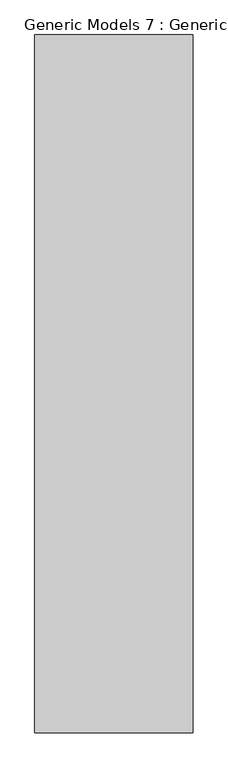
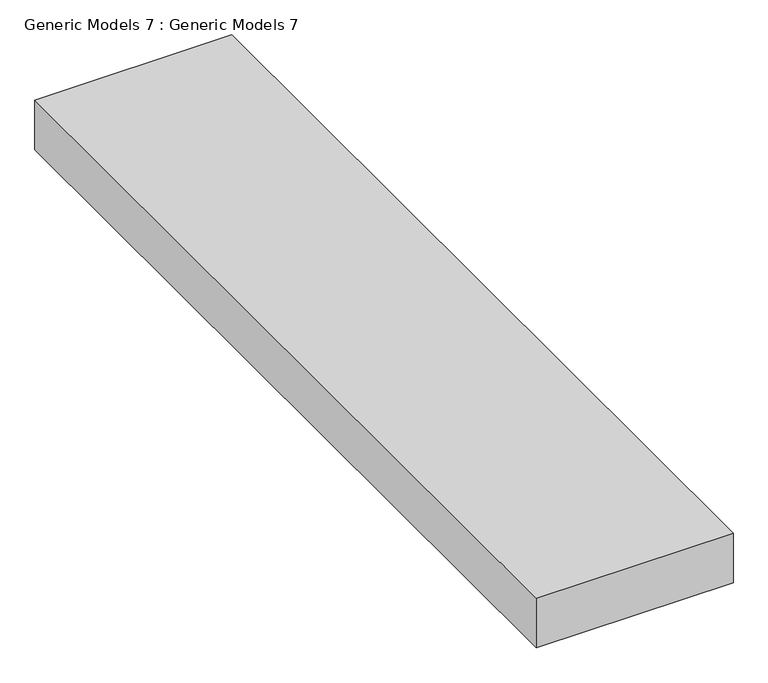
"""IFC4 building model written with IfcOpenShell, lengths in millimetres: proxy geometry, Generic Models 7 : Generic Models 7."""

from ifc_helpers import new_model, si_unit, frame, origin, place, context, project, spatial, polyline, outline, extrude, source, transform, mapped, element, save


def generic_models_7_generic_models_7_79cca6d0(model_context):
    return source(origin(), model_context, "Body", "SweptSolid", [
        extrude(outline(polyline([(-8624.9161422, -4183.027471), (-9196.4161422, -4183.027471), (-9196.4161422, -1660.6643401), (-8624.9161422, -1660.6643401), (-8624.9161422, -4183.027471)])), frame((0.0, 0.0, 2477.8166854), z_axis=(0.0, 0.0, 1.0), x_axis=(1.0, 0.0, 0.0)), (0.0, 0.0, 1.0), 152.4),
    ])


if __name__ == "__main__":
    model = new_model("IFC4")
    model_context = context("Model", 3, world=origin())
    ifc_project = project(units=[si_unit("LENGTHUNIT", "METRE", prefix="MILLI")], contexts=[model_context])
    site = spatial("IfcSite", under=ifc_project)
    building = spatial("IfcBuilding", under=site)
    placement = place(None, origin())
    generic_models_7_generic_models_7_shape = generic_models_7_generic_models_7_79cca6d0(model_context)
    element("IfcBuildingElementProxy", 1, Name="Generic Models 7 : Generic Models 7", ObjectType="Generic Models 7 : Generic Models 7", at=placement, inside=building, context=model_context, shape_type="MappedRepresentation", body=[
        mapped(generic_models_7_generic_models_7_shape, transform((0.0, 0.0, 0.0), x_axis=(1.0, 0.0, 0.0), y_axis=(0.0, 1.0, 0.0), z_axis=(0.0, 0.0, 1.0))),
    ])
    save(model, "model.ifc")
